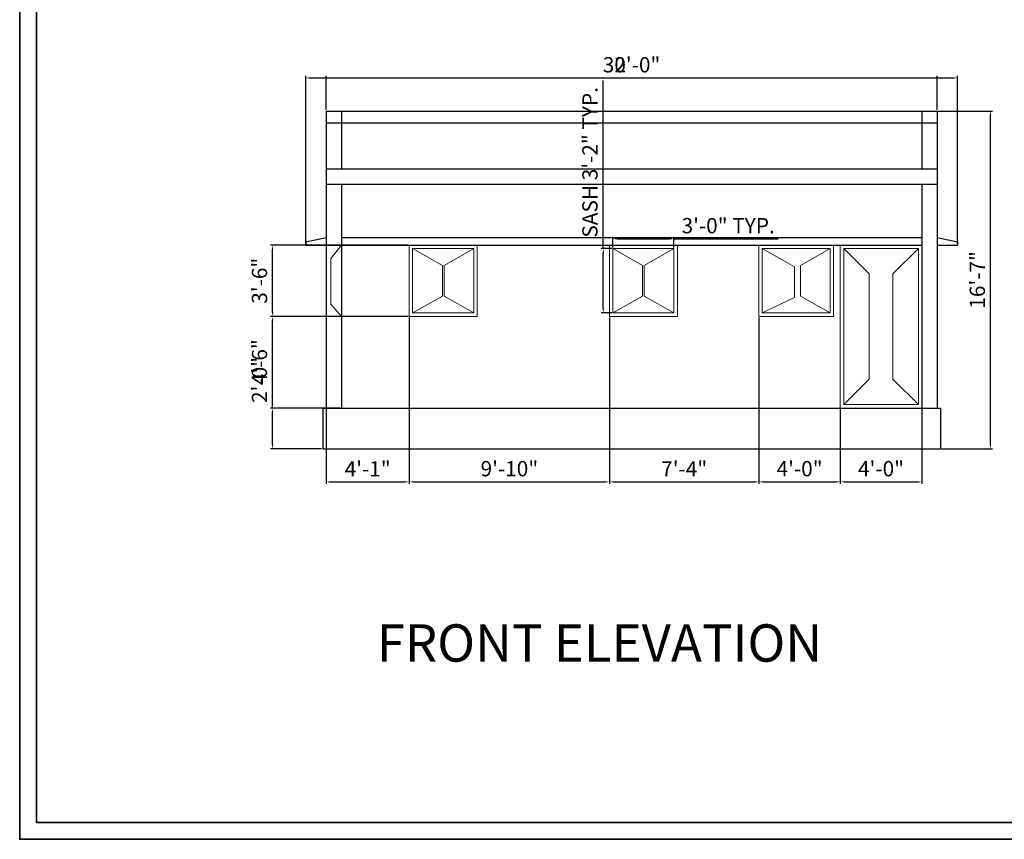
# Model space of a CAD drawing. Units: inches. Extents: x 2413 to 4117, y 1127 to 2321.
# Tile 1 of 5: x 2413 to 2993, y 1127 to 1610. Entities that reach past the tile are written whole.
import ezdxf

# ---------------------------------------------------------------- set-up
doc = ezdxf.new("R2010")
doc.units = ezdxf.units.IN
doc.linetypes.add('ACAD_ISO03W100', pattern=[30, 12, -18])
doc.layers.get('Defpoints').update_dxf_attribs({"linetype": 'ACAD_ISO03W100'})
for name, color, linetype, lineweight in [('A-ANNO-DIMS', 2, 'Continuous', 18), ('A-ANNO-TITL', 7, 'Continuous', 30), ('A-ANNO-TTLB', 7, 'Continuous', 35), ('A-DOOR', 3, 'Continuous', 20), ('A-ELEV', 7, 'Continuous', 25), ('A-FLOR', 7, 'Continuous', 30), ('A-GLAZ', 4, 'Continuous', 18), ('A-ROOF', 7, 'Continuous', 30)]:
    doc.layers.add(name, color=color, linetype=linetype, lineweight=lineweight)
doc.styles.get("Standard").update_dxf_attribs({"font": 'arial.ttf'})
doc.dimstyles.new('ISO-25', dxfattribs={"dimtxt": 9, "dimasz": 2.5, "dimexe": 1.25, "dimexo": 0.625, "dimgap": 2, "dimtad": 1, "dimdec": 1, "dimlunit": 4, "dimtxsty": 'Standard', "dimcen": 2.5, "dimazin": 0, "dimtfac": 1, "dimtdec": 1, "dimtmove": 0, "dimatfit": 3, "dimfxl": 1, "dimarcsym": 0})

# ---------------------------------------------------------------- blocks, each defined once
blk = doc.blocks.new('WIN-CASEMENT-36-SASH-ELEV')
for p, q in [((0, 38), (36, 38)), ((0, 38), (0, 0)), ((0, 38), (17.5, 28)), ((18.5, 28), (36, 38)), ((36, 38), (36, 0)), ((17.5, 28), (17.5, 10)), ((18.5, 28), (18.5, 10)), ((0, 0), (17.5, 10)), ((18.5, 10), (36, 0)), ((0, 0), (36, 0))]:
    blk.add_line(p, q)
blk = doc.blocks.new('*D24')
at = {"layer": 'A-ANNO-DIMS', "color": 0, "lineweight": -2, "transparency": 16777216}
for p, q in [((2756.47, 1475.03), (2756.47, 1574.08)), ((2761.54, 1475.03), (2755.22, 1475.03)), ((2756.47, 1439.53), (2756.47, 1472.53)), ((2761.54, 1437.03), (2755.22, 1437.03))]:
    blk.add_line(p, q, dxfattribs=at)
at = {"layer": 'A-ANNO-DIMS', "color": 0, "transparency": 16777216}
for points in [[(2756.05, 1472.53), (2756.89, 1472.53), (2756.47, 1475.03)], [(2756.05, 1439.53), (2756.89, 1439.53), (2756.47, 1437.03)]]:
    blk.add_solid(points, dxfattribs=at)
at = {"layer": 'Defpoints', "color": 0, "transparency": 16777216}
for p in [(2756.47, 1475.03), (2762.17, 1475.03), (2762.17, 1437.03)]:
    blk.add_point(p, dxfattribs=at)
at = {"layer": 'A-ANNO-DIMS', "color": 0, "transparency": 16777216, "insert": (2749.81, 1525.81), "char_height": 9, "attachment_point": 5, "rotation": 90}
blk.add_mtext('SASH 3\'-2" TYP.', dxfattribs=at)
blk = doc.blocks.new('*D25')
at = {"layer": 'A-ANNO-DIMS', "color": 0, "lineweight": -2, "transparency": 16777216}
for p, q in [((2762.17, 1475.66), (2762.17, 1481.98)), ((2764.67, 1480.73), (2795.67, 1480.73)), ((2798.17, 1475.66), (2798.17, 1481.98)), ((2798.17, 1480.73), (2859.52, 1480.73))]:
    blk.add_line(p, q, dxfattribs=at)
at = {"layer": 'A-ANNO-DIMS', "color": 0, "transparency": 16777216}
for points in [[(2764.67, 1481.15), (2764.67, 1480.32), (2762.17, 1480.73)], [(2795.67, 1481.15), (2795.67, 1480.32), (2798.17, 1480.73)]]:
    blk.add_solid(points, dxfattribs=at)
at = {"layer": 'Defpoints', "color": 0, "transparency": 16777216}
for p in [(2798.17, 1480.73), (2762.17, 1475.03), (2798.17, 1475.03)]:
    blk.add_point(p, dxfattribs=at)
at = {"layer": 'A-ANNO-DIMS', "color": 0, "transparency": 16777216, "insert": (2830.1, 1487.33), "char_height": 9, "attachment_point": 5}
blk.add_mtext('3\'-0" TYP.', dxfattribs=at)
blk = doc.blocks.new('*D66')
at = {"layer": 'A-ANNO-DIMS', "color": 0, "lineweight": -2, "transparency": 16777216}
for p, q in [((2581.17, 1477.66), (2581.17, 1576.78)), ((2583.67, 1575.53), (2962.67, 1575.53)), ((2965.17, 1477.66), (2965.17, 1576.78))]:
    blk.add_line(p, q, dxfattribs=at)
at = {"layer": 'A-ANNO-DIMS', "color": 0, "transparency": 16777216}
for points in [[(2583.67, 1575.95), (2583.67, 1575.12), (2581.17, 1575.53)], [(2962.67, 1575.95), (2962.67, 1575.12), (2965.17, 1575.53)]]:
    blk.add_solid(points, dxfattribs=at)
at = {"layer": 'Defpoints', "color": 0, "transparency": 16777216}
for p in [(2965.17, 1575.53), (2581.17, 1477.03), (2965.17, 1477.03)]:
    blk.add_point(p, dxfattribs=at)
at = {"layer": 'A-ANNO-DIMS', "color": 0, "transparency": 16777216, "insert": (2773.17, 1582.13), "char_height": 9, "attachment_point": 5}
blk.add_mtext('32\'-0"', dxfattribs=at)
blk = doc.blocks.new('*D67')
at = {"layer": 'A-ANNO-DIMS', "color": 0, "lineweight": -2, "transparency": 16777216}
for p, q in [((2953.79, 1556.03), (2985.92, 1556.03)), ((2984.67, 1359.53), (2984.67, 1553.53)), ((2955.79, 1357.03), (2985.92, 1357.03))]:
    blk.add_line(p, q, dxfattribs=at)
at = {"layer": 'A-ANNO-DIMS', "color": 0, "transparency": 16777216}
for points in [[(2984.25, 1553.53), (2985.09, 1553.53), (2984.67, 1556.03)], [(2984.25, 1359.53), (2985.09, 1359.53), (2984.67, 1357.03)]]:
    blk.add_solid(points, dxfattribs=at)
at = {"layer": 'Defpoints', "color": 0, "transparency": 16777216}
for p in [(2953.17, 1556.03), (2984.67, 1556.03), (2955.17, 1357.03)]:
    blk.add_point(p, dxfattribs=at)
at = {"layer": 'A-ANNO-DIMS', "color": 0, "transparency": 16777216, "insert": (2978.07, 1456.53), "char_height": 9, "attachment_point": 5, "rotation": 90}
blk.add_mtext('16\'-7"', dxfattribs=at)
blk = doc.blocks.new('*D68')
at = {"layer": 'A-ANNO-DIMS', "color": 0, "lineweight": -2, "transparency": 16777216}
for p, q in [((2593.17, 1556.66), (2593.17, 1576.78)), ((2595.67, 1575.53), (2950.67, 1575.53)), ((2953.17, 1556.66), (2953.17, 1576.78))]:
    blk.add_line(p, q, dxfattribs=at)
at = {"layer": 'A-ANNO-DIMS', "color": 0, "transparency": 16777216}
for points in [[(2595.67, 1575.95), (2595.67, 1575.12), (2593.17, 1575.53)], [(2950.67, 1575.95), (2950.67, 1575.12), (2953.17, 1575.53)]]:
    blk.add_solid(points, dxfattribs=at)
at = {"layer": 'Defpoints', "color": 0, "transparency": 16777216}
for p in [(2953.17, 1575.53), (2593.17, 1556.03), (2953.17, 1556.03)]:
    blk.add_point(p, dxfattribs=at)
at = {"layer": 'A-ANNO-DIMS', "color": 0, "transparency": 16777216, "insert": (2773.17, 1582.13), "char_height": 9, "attachment_point": 5}
blk.add_mtext('30\'-0"', dxfattribs=at)
blk = doc.blocks.new('*D69')
at = {"layer": 'A-ANNO-DIMS', "color": 0, "lineweight": -2, "transparency": 16777216}
for p, q in [((2642.17, 1434.41), (2642.17, 1336.28)), ((2593.17, 1380.41), (2593.17, 1336.28)), ((2595.67, 1337.53), (2639.67, 1337.53))]:
    blk.add_line(p, q, dxfattribs=at)
at = {"layer": 'A-ANNO-DIMS', "color": 0, "transparency": 16777216}
for points in [[(2595.67, 1337.95), (2595.67, 1337.12), (2593.17, 1337.53)], [(2639.67, 1337.95), (2639.67, 1337.12), (2642.17, 1337.53)]]:
    blk.add_solid(points, dxfattribs=at)
at = {"layer": 'Defpoints', "color": 0, "transparency": 16777216}
for p in [(2642.17, 1435.03), (2593.17, 1381.03), (2642.17, 1337.53)]:
    blk.add_point(p, dxfattribs=at)
at = {"layer": 'A-ANNO-DIMS', "color": 0, "transparency": 16777216, "insert": (2617.67, 1344.05), "char_height": 9, "attachment_point": 5}
blk.add_mtext('4\'-1"', dxfattribs=at)
blk = doc.blocks.new('*D70')
at = {"layer": 'A-ANNO-DIMS', "color": 0, "lineweight": -2, "transparency": 16777216}
for p, q in [((2642.17, 1434.41), (2642.17, 1336.28)), ((2760.17, 1434.41), (2760.17, 1336.28)), ((2644.67, 1337.53), (2757.67, 1337.53))]:
    blk.add_line(p, q, dxfattribs=at)
at = {"layer": 'A-ANNO-DIMS', "color": 0, "transparency": 16777216}
for points in [[(2644.67, 1337.95), (2644.67, 1337.12), (2642.17, 1337.53)], [(2757.67, 1337.95), (2757.67, 1337.12), (2760.17, 1337.53)]]:
    blk.add_solid(points, dxfattribs=at)
at = {"layer": 'Defpoints', "color": 0, "transparency": 16777216}
for p in [(2642.17, 1435.03), (2760.17, 1435.03), (2760.17, 1337.53)]:
    blk.add_point(p, dxfattribs=at)
at = {"layer": 'A-ANNO-DIMS', "color": 0, "transparency": 16777216, "insert": (2701.17, 1344.13), "char_height": 9, "attachment_point": 5}
blk.add_mtext('9\'-10"', dxfattribs=at)
blk = doc.blocks.new('*D71')
at = {"layer": 'A-ANNO-DIMS', "color": 0, "lineweight": -2, "transparency": 16777216}
for p, q in [((2760.17, 1434.41), (2760.17, 1336.28)), ((2848.17, 1434.41), (2848.17, 1336.28)), ((2762.67, 1337.53), (2845.67, 1337.53))]:
    blk.add_line(p, q, dxfattribs=at)
at = {"layer": 'A-ANNO-DIMS', "color": 0, "transparency": 16777216}
for points in [[(2762.67, 1337.95), (2762.67, 1337.12), (2760.17, 1337.53)], [(2845.67, 1337.95), (2845.67, 1337.12), (2848.17, 1337.53)]]:
    blk.add_solid(points, dxfattribs=at)
at = {"layer": 'Defpoints', "color": 0, "transparency": 16777216}
for p in [(2760.17, 1435.03), (2848.17, 1435.03), (2848.17, 1337.53)]:
    blk.add_point(p, dxfattribs=at)
at = {"layer": 'A-ANNO-DIMS', "color": 0, "transparency": 16777216, "insert": (2804.17, 1344.03), "char_height": 9, "attachment_point": 5}
blk.add_mtext('7\'-4"', dxfattribs=at)
blk = doc.blocks.new('*D72')
at = {"layer": 'A-ANNO-DIMS', "color": 0, "lineweight": -2, "transparency": 16777216}
for p, q in [((2848.17, 1434.41), (2848.17, 1336.28)), ((2896.17, 1380.41), (2896.17, 1336.28)), ((2850.67, 1337.53), (2893.67, 1337.53))]:
    blk.add_line(p, q, dxfattribs=at)
at = {"layer": 'A-ANNO-DIMS', "color": 0, "transparency": 16777216}
for points in [[(2850.67, 1337.95), (2850.67, 1337.12), (2848.17, 1337.53)], [(2893.67, 1337.95), (2893.67, 1337.12), (2896.17, 1337.53)]]:
    blk.add_solid(points, dxfattribs=at)
at = {"layer": 'Defpoints', "color": 0, "transparency": 16777216}
for p in [(2848.17, 1435.03), (2896.17, 1381.03), (2896.17, 1337.53)]:
    blk.add_point(p, dxfattribs=at)
at = {"layer": 'A-ANNO-DIMS', "color": 0, "transparency": 16777216, "insert": (2872.17, 1344.13), "char_height": 9, "attachment_point": 5}
blk.add_mtext('4\'-0"', dxfattribs=at)
blk = doc.blocks.new('*D73')
at = {"layer": 'A-ANNO-DIMS', "color": 0, "lineweight": -2, "transparency": 16777216}
for p, q in [((2896.17, 1380.41), (2896.17, 1336.28)), ((2944.17, 1380.41), (2944.17, 1336.28)), ((2898.67, 1337.53), (2941.67, 1337.53))]:
    blk.add_line(p, q, dxfattribs=at)
at = {"layer": 'A-ANNO-DIMS', "color": 0, "transparency": 16777216}
for points in [[(2898.67, 1337.95), (2898.67, 1337.12), (2896.17, 1337.53)], [(2941.67, 1337.95), (2941.67, 1337.12), (2944.17, 1337.53)]]:
    blk.add_solid(points, dxfattribs=at)
at = {"layer": 'Defpoints', "color": 0, "transparency": 16777216}
for p in [(2896.17, 1381.03), (2944.17, 1381.03), (2944.17, 1337.53)]:
    blk.add_point(p, dxfattribs=at)
at = {"layer": 'A-ANNO-DIMS', "color": 0, "transparency": 16777216, "insert": (2920.17, 1344.13), "char_height": 9, "attachment_point": 5}
blk.add_mtext('4\'-0"', dxfattribs=at)
blk = doc.blocks.new('*D74')
at = {"layer": 'A-ANNO-DIMS', "color": 0, "lineweight": -2, "transparency": 16777216}
for p, q in [((2641.54, 1477.03), (2560.42, 1477.03)), ((2561.67, 1437.53), (2561.67, 1474.53)), ((2641.54, 1435.03), (2560.42, 1435.03))]:
    blk.add_line(p, q, dxfattribs=at)
at = {"layer": 'A-ANNO-DIMS', "color": 0, "transparency": 16777216}
for points in [[(2561.25, 1474.53), (2562.09, 1474.53), (2561.67, 1477.03)], [(2561.25, 1437.53), (2562.09, 1437.53), (2561.67, 1435.03)]]:
    blk.add_solid(points, dxfattribs=at)
at = {"layer": 'Defpoints', "color": 0, "transparency": 16777216}
for p in [(2561.67, 1477.03), (2642.17, 1477.03), (2642.17, 1435.03)]:
    blk.add_point(p, dxfattribs=at)
at = {"layer": 'A-ANNO-DIMS', "color": 0, "transparency": 16777216, "insert": (2555.07, 1456.03), "char_height": 9, "attachment_point": 5, "rotation": 90}
blk.add_mtext('3\'-6"', dxfattribs=at)
blk = doc.blocks.new('*D75')
at = {"layer": 'A-ANNO-DIMS', "color": 0, "lineweight": -2, "transparency": 16777216}
for p, q in [((2641.54, 1435.03), (2560.42, 1435.03)), ((2561.67, 1383.53), (2561.67, 1432.53)), ((2601.54, 1381.03), (2560.42, 1381.03))]:
    blk.add_line(p, q, dxfattribs=at)
at = {"layer": 'A-ANNO-DIMS', "color": 0, "transparency": 16777216}
for points in [[(2561.25, 1432.53), (2562.09, 1432.53), (2561.67, 1435.03)], [(2561.25, 1383.53), (2562.09, 1383.53), (2561.67, 1381.03)]]:
    blk.add_solid(points, dxfattribs=at)
at = {"layer": 'Defpoints', "color": 0, "transparency": 16777216}
for p in [(2561.67, 1435.03), (2642.17, 1435.03), (2602.17, 1381.03)]:
    blk.add_point(p, dxfattribs=at)
at = {"layer": 'A-ANNO-DIMS', "color": 0, "transparency": 16777216, "insert": (2555.07, 1408.03), "char_height": 9, "attachment_point": 5, "rotation": 90}
blk.add_mtext('4\'-6"', dxfattribs=at)
blk = doc.blocks.new('*D76')
at = {"layer": 'A-ANNO-DIMS', "color": 0, "lineweight": -2, "transparency": 16777216}
for p, q in [((2561.67, 1381.03), (2561.67, 1411.61)), ((2590.54, 1381.03), (2560.42, 1381.03)), ((2561.67, 1359.53), (2561.67, 1378.53)), ((2590.54, 1357.03), (2560.42, 1357.03))]:
    blk.add_line(p, q, dxfattribs=at)
at = {"layer": 'A-ANNO-DIMS', "color": 0, "transparency": 16777216}
for points in [[(2561.25, 1378.53), (2562.09, 1378.53), (2561.67, 1381.03)], [(2561.25, 1359.53), (2562.09, 1359.53), (2561.67, 1357.03)]]:
    blk.add_solid(points, dxfattribs=at)
at = {"layer": 'Defpoints', "color": 0, "transparency": 16777216}
for p in [(2561.67, 1381.03), (2591.17, 1381.03), (2591.17, 1357.03)]:
    blk.add_point(p, dxfattribs=at)
at = {"layer": 'A-ANNO-DIMS', "color": 0, "transparency": 16777216, "insert": (2555.07, 1397.57), "char_height": 9, "attachment_point": 5, "rotation": 90}
blk.add_mtext('2\'-0"', dxfattribs=at)

msp = doc.modelspace()

# ---------------------------------------------------------------- linework, layer by layer
at = {"layer": 'A-ANNO-TTLB'}
for points in [[(2412.62, 2321.32), (4117.04, 2321.32), (4117.04, 1126.9), (2412.62, 1126.9)], [(2422.62, 2311.32), (4107.04, 2311.32), (4107.04, 1136.9), (2422.62, 1136.9)]]:
    msp.add_lwpolyline(points, close=True, dxfattribs=at)
at = {"layer": 'A-DOOR'}
for p, q in [((2896.17, 1477.03), (2896.17, 1381.03)), ((2896.17, 1477.03), (2944.17, 1477.03)), ((2898.17, 1475.03), (2913.17, 1460.03)), ((2898.17, 1475.03), (2942.17, 1475.03)), ((2898.17, 1475.03), (2898.17, 1383.03)), ((2927.17, 1460.03), (2942.17, 1475.03)), ((2942.17, 1475.03), (2942.17, 1383.03)), ((2913.17, 1460.03), (2913.17, 1398.03)), ((2927.17, 1460.03), (2927.17, 1398.03)), ((2898.17, 1383.03), (2913.17, 1398.03)), ((2927.17, 1398.03), (2942.17, 1383.03)), ((2898.17, 1383.03), (2942.17, 1383.03)), ((2898.17, 1383.03), (2942.17, 1383.03))]:
    msp.add_line(p, q, dxfattribs=at)
at = {"layer": 'A-ELEV'}
for p, q in [((2593.17, 1556.03), (2593.17, 1383.03)), ((2602.17, 1556.03), (2602.17, 1522.03)), ((2944.17, 1556.03), (2944.17, 1522.03)), ((2953.17, 1556.03), (2953.17, 1381.03)), ((2602.17, 1513.03), (2602.17, 1381.03)), ((2944.17, 1513.03), (2944.17, 1381.03)), ((2581.17, 1479.03), (2593.17, 1481.53)), ((2602.17, 1481.53), (2944.17, 1481.53)), ((2953.17, 1481.53), (2965.17, 1479.03)), ((2581.17, 1479.03), (2581.17, 1477.03)), ((2581.17, 1477.03), (2593.17, 1477.03)), ((2593.17, 1477.03), (2944.17, 1477.03)), ((2953.17, 1477.03), (2965.17, 1477.03)), ((2953.17, 1477.03), (2965.17, 1477.03)), ((2965.17, 1479.03), (2965.17, 1477.03)), ((2593.17, 1383.03), (2593.17, 1381.03))]:
    msp.add_line(p, q, dxfattribs=at)
at = {"layer": 'A-FLOR'}
for p, q in [((2591.17, 1381.03), (2955.17, 1381.03)), ((2591.17, 1381.03), (2591.17, 1357.03)), ((2828.17, 1381.03), (2838.17, 1381.03)), ((2953.17, 1381.03), (2955.17, 1381.03)), ((2955.17, 1381.03), (2955.17, 1357.03)), ((2591.17, 1357.03), (2955.17, 1357.03)), ((2953.17, 1357.03), (2955.17, 1357.03))]:
    msp.add_line(p, q, dxfattribs=at)
at = {"layer": 'A-GLAZ'}
for p, q in [((2602.17, 1477.03), (2595.99, 1469.18)), ((2642.17, 1477.03), (2642.17, 1435.03)), ((2682.17, 1477.03), (2682.17, 1435.03)), ((2760.17, 1477.03), (2760.17, 1435.03)), ((2760.17, 1477.03), (2800.17, 1477.03)), ((2800.17, 1477.03), (2800.17, 1435.03)), ((2848.17, 1477.03), (2848.17, 1435.03)), ((2848.17, 1477.03), (2848.17, 1435.03)), ((2848.17, 1477.03), (2892.17, 1477.03)), ((2850.17, 1475.03), (2869.17, 1464.17)), ((2850.17, 1475.03), (2890.17, 1475.03)), ((2850.17, 1475.03), (2850.17, 1437.03)), ((2872.67, 1465.03), (2890.17, 1475.03)), ((2890.17, 1475.03), (2890.17, 1437.03)), ((2892.17, 1477.03), (2892.17, 1435.03)), ((2595.99, 1469.18), (2595.99, 1442.14)), ((2869.17, 1464.17), (2869.17, 1446.17)), ((2872.67, 1465.03), (2872.67, 1447.03)), ((2850.17, 1437.03), (2869.17, 1446.17)), ((2872.67, 1447.03), (2890.17, 1437.03)), ((2595.99, 1442.14), (2602.17, 1435.03)), ((2593.17, 1435.03), (2602.17, 1435.03)), ((2642.17, 1435.03), (2682.17, 1435.03)), ((2760.17, 1435.03), (2800.17, 1435.03)), ((2848.17, 1435.03), (2892.17, 1435.03)), ((2850.17, 1437.03), (2890.17, 1437.03))]:
    msp.add_line(p, q, dxfattribs=at)
at = {"layer": 'A-ROOF'}
for p, q in [((2593.17, 1556.03), (2953.17, 1556.03)), ((2593.17, 1549.03), (2953.17, 1549.03)), ((2593.17, 1522.03), (2953.17, 1522.03)), ((2593.17, 1513.03), (2953.17, 1513.03))]:
    msp.add_line(p, q, dxfattribs=at)

# ---------------------------------------------------------------- block references
at = {"layer": 'A-GLAZ'}
for p in [(2644.17, 1437.03), (2762.17, 1437.03)]:
    msp.add_blockref('WIN-CASEMENT-36-SASH-ELEV', p, dxfattribs=at)

# ---------------------------------------------------------------- texts
at = {"layer": 'A-ANNO-TITL'}
msp.add_text('FRONT ELEVATION', height=22.0248, dxfattribs=at).set_placement((2622.99, 1231.56))

# ---------------------------------------------------------------- dimensions: what is measured, and where the dimension line sits
at = {"layer": 'A-ANNO-DIMS'}
for base, p1, p2, picture, middle in [((2965.17, 1575.53), (2581.17, 1477.03), (2965.17, 1477.03), '*D66', (2773.17, 1582.13)), ((2953.17, 1575.53), (2593.17, 1556.03), (2953.17, 1556.03), '*D68', (2773.17, 1582.13)), ((2642.17, 1337.53), (2593.17, 1381.03), (2642.17, 1435.03), '*D69', (2617.67, 1344.05)), ((2760.17, 1337.53), (2642.17, 1435.03), (2760.17, 1435.03), '*D70', (2701.17, 1344.13)), ((2848.17, 1337.53), (2760.17, 1435.03), (2848.17, 1435.03), '*D71', (2804.17, 1344.03)), ((2896.17, 1337.53), (2848.17, 1435.03), (2896.17, 1381.03), '*D72', (2872.17, 1344.13)), ((2944.17, 1337.53), (2896.17, 1381.03), (2944.17, 1381.03), '*D73', (2920.17, 1344.13))]:
    dim = msp.add_linear_dim(base=base, p1=p1, p2=p2, dimstyle='ISO-25', override={"dimdec": 1, "dimlfac": 1, "dimrnd": 0, "dimzin": 1, "dimdsep": 46, "dimlunit": 4, "dimfrac": 2}, dxfattribs=at)
    dim.commit()
    dim.dimension.update_dxf_attribs({"geometry": picture, "text_midpoint": middle})
dim = msp.add_linear_dim(base=(2756.47, 1475.03), p1=(2762.17, 1437.03), p2=(2762.17, 1475.03), angle=90, text='SASH <> TYP.', dimstyle='ISO-25', override={"dimdec": 1, "dimlfac": 1, "dimrnd": 0, "dimzin": 1, "dimdsep": 46, "dimlunit": 4, "dimfrac": 2}, dxfattribs=at)
dim.commit()
dim.dimension.update_dxf_attribs({"geometry": '*D24', "text_midpoint": (2749.81, 1525.81)})
for base, p1, p2, picture, middle in [((2984.67, 1556.03), (2955.17, 1357.03), (2953.17, 1556.03), '*D67', (2978.07, 1456.53)), ((2561.67, 1477.03), (2642.17, 1435.03), (2642.17, 1477.03), '*D74', (2555.07, 1456.03)), ((2561.67, 1435.03), (2602.17, 1381.03), (2642.17, 1435.03), '*D75', (2555.07, 1408.03)), ((2561.67, 1381.03), (2591.17, 1357.03), (2591.17, 1381.03), '*D76', (2555.07, 1397.57))]:
    dim = msp.add_linear_dim(base=base, p1=p1, p2=p2, angle=90, dimstyle='ISO-25', override={"dimdec": 1, "dimlfac": 1, "dimrnd": 0, "dimzin": 1, "dimdsep": 46, "dimlunit": 4, "dimfrac": 2}, dxfattribs=at)
    dim.commit()
    dim.dimension.update_dxf_attribs({"geometry": picture, "text_midpoint": middle})
dim = msp.add_linear_dim(base=(2798.17, 1480.73), p1=(2762.17, 1475.03), p2=(2798.17, 1475.03), text='<> TYP.', dimstyle='ISO-25', override={"dimdec": 1, "dimlfac": 1, "dimrnd": 0, "dimzin": 1, "dimdsep": 46, "dimlunit": 4, "dimfrac": 2}, dxfattribs=at)
dim.commit()
dim.dimension.update_dxf_attribs({"geometry": '*D25', "text_midpoint": (2830.1, 1487.33)})

doc.saveas('drawing.dxf')
